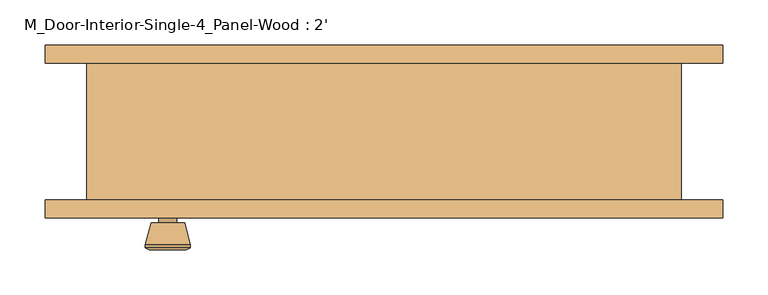
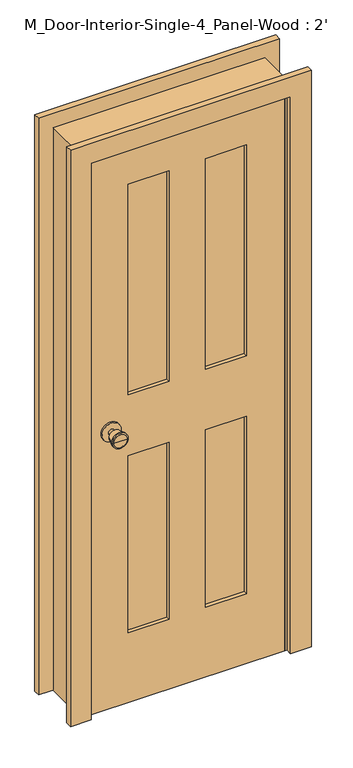
"""IFC4 building model written with IfcOpenShell, lengths in millimetres: door geometry, M_Door-Interior-Single-4_Panel-Wood : 2'."""

from ifc_helpers import new_model, si_unit, point, frame, frame_2d, origin, place, context, project, spatial, polyline, circle_curve, trimmed, segment, composite_curve, outline, extrude, faceted_brep, source, transform, mapped, element, save
from ifc_brep_helpers import plane_surface, cylinder_surface, revolved_surface, advanced_brep


def m_door_interior_single_4_panel_wood_2_b7882c25(model_context):
    return source(origin(), model_context, "Body", "SolidModel", [
        advanced_brep(
        [(-239.8, -32.025, 914.4), (-249.8, -32.025, 914.4), (-229.8, -32.025, 914.4), (-219.3241324, 16.975, 914.4), (-260.2758676, 16.975, 914.4), (-239.8, 16.975, 914.4), (-214.8, 15.1471319, 914.4), (-264.8, 15.1471319, 914.4), (-214.8, 11.6834537, 914.4), (-264.8, 11.6834537, 914.4), (-221.163764, -13.025, 914.4), (-258.436236, -13.025, 914.4), (-229.8, -13.025, 914.4), (-249.8, -13.025, 914.4)],
        [
            (0, 1),
            (1, 2, circle_curve(frame((-239.8, -32.025, 914.4), z_axis=(0.0, -1.0, 0.0), x_axis=(-1.0, 0.0, 0.0)), 10.0)),
            (2, 0),
            (2, 1, circle_curve(frame((-239.8, -32.025, 914.4), z_axis=(0.0, -1.0, 0.0), x_axis=(-1.0, 0.0, 0.0)), 10.0)),
            (3, 4, circle_curve(frame((-239.8, 16.975, 914.4), z_axis=(0.0, 1.0, 0.0), x_axis=(-1.0, 0.0, 0.0)), 20.4758676)),
            (4, 5),
            (5, 3),
            (4, 3, circle_curve(frame((-239.8, 16.975, 914.4), z_axis=(0.0, 1.0, 0.0), x_axis=(-1.0, 0.0, 0.0)), 20.4758676)),
            (6, 7, circle_curve(frame((-239.8, 15.1471319, 914.4), z_axis=(0.0, 1.0, 0.0), x_axis=(-1.0, 0.0, 0.0)), 25.0)),
            (7, 4),
            (3, 6),
            (7, 6, circle_curve(frame((-239.8, 15.1471319, 914.4), z_axis=(0.0, 1.0, 0.0), x_axis=(-1.0, 0.0, 0.0)), 25.0)),
            (8, 9, circle_curve(frame((-239.8, 11.6834537, 914.4), z_axis=(0.0, 1.0, 0.0), x_axis=(-1.0, 0.0, 0.0)), 25.0)),
            (9, 7),
            (6, 8),
            (9, 8, circle_curve(frame((-239.8, 11.6834537, 914.4), z_axis=(0.0, 1.0, 0.0), x_axis=(-1.0, 0.0, 0.0)), 25.0)),
            (10, 11, circle_curve(frame((-239.8, -13.025, 914.4), z_axis=(0.0, 1.0, 0.0), x_axis=(-1.0, 0.0, 0.0)), 18.636236)),
            (11, 9),
            (8, 10),
            (11, 10, circle_curve(frame((-239.8, -13.025, 914.4), z_axis=(0.0, 1.0, 0.0), x_axis=(-1.0, 0.0, 0.0)), 18.636236)),
            (12, 13, circle_curve(frame((-239.8, -13.025, 914.4), z_axis=(0.0, 1.0, 0.0), x_axis=(-1.0, 0.0, 0.0)), 10.0)),
            (13, 11),
            (10, 12),
            (13, 12, circle_curve(frame((-239.8, -13.025, 914.4), z_axis=(0.0, 1.0, 0.0), x_axis=(-1.0, 0.0, 0.0)), 10.0)),
            (1, 13),
            (12, 2),
        ],
        [
            plane_surface(frame((-239.8, -32.025, 914.4), z_axis=(0.0, -1.0, 0.0), x_axis=(-1.0, 0.0, 0.0))),
            plane_surface(frame((-239.8, 16.975, 914.4), z_axis=(0.0, 1.0, 0.0), x_axis=(-1.0, 0.0, 0.0))),
            revolved_surface(polyline([(-260.2758676, 16.975, 914.4), (-264.8, 15.1471319, 914.4)]), (-239.8, -32.025, 914.4), (0.0, -1.0, 0.0)),
            cylinder_surface(frame((-239.8, -32.025, 914.4), z_axis=(0.0, -1.0, 0.0), x_axis=(-1.0, 0.0, 0.0)), 25.0),
            revolved_surface(polyline([(-264.8, 11.6834537, 914.4), (-258.436236, -13.025, 914.4)]), (-239.8, -32.025, 914.4), (0.0, -1.0, 0.0)),
            plane_surface(frame((-239.8, -13.025, 914.4), z_axis=(0.0, -1.0, 0.0), x_axis=(-1.0, 0.0, 0.0))),
            cylinder_surface(frame((-239.8, -32.025, 914.4), z_axis=(0.0, -1.0, 0.0), x_axis=(-1.0, 0.0, 0.0)), 10.0),
        ],
        [
            (0, [[1, 2, 3]]),
            (0, [[-3, 4, -1]]),
            (1, [[5, 6, 7]]),
            (1, [[8, -7, -6]]),
            (2, [[9, 10, -5, 11]]),
            (2, [[12, -11, -8, -10]]),
            (3, [[13, 14, -9, 15]]),
            (3, [[16, -15, -12, -14]]),
            (4, [[17, 18, -13, 19]]),
            (4, [[20, -19, -16, -18]]),
            (5, [[21, 22, -17, 23]]),
            (5, [[24, -23, -20, -22]]),
            (6, [[-2, 25, -21, 26]]),
            (6, [[-4, -26, -24, -25]]),
        ],
    ),
        extrude(outline(composite_curve([segment(trimmed(circle_curve(frame_2d((914.4, -239.8)), 30.0), [point((914.4, -269.8))], [point((914.4, -209.8))], False, "CARTESIAN"), True, "CONTINUOUS"), segment(trimmed(circle_curve(frame_2d((914.4, -239.8)), 30.0), [point((914.4, -209.8))], [point((914.4, -269.8))], False, "CARTESIAN"), True, "CONTINUOUS")], self_intersect=False)), frame((0.0, -38.025, 0.0), z_axis=(0.0, 1.0, 0.0), x_axis=(0.0, 0.0, 1.0)), (0.0, 0.0, 1.0), 6.0),
        advanced_brep(
        [(-239.8, -79.025, 914.4), (-229.8, -79.025, 914.4), (-249.8, -79.025, 914.4), (-219.3241324, -128.025, 914.4), (-239.8, -128.025, 914.4), (-260.2758676, -128.025, 914.4), (-214.8, -126.1971319, 914.4), (-264.8, -126.1971319, 914.4), (-214.8, -122.7334537, 914.4), (-264.8, -122.7334537, 914.4), (-221.163764, -98.025, 914.4), (-258.436236, -98.025, 914.4), (-229.8, -98.025, 914.4), (-249.8, -98.025, 914.4)],
        [
            (0, 1),
            (1, 2, circle_curve(frame((-239.8, -79.025, 914.4), z_axis=(0.0, 1.0, 0.0), x_axis=(-1.0, 0.0, 0.0)), 10.0)),
            (2, 0),
            (2, 1, circle_curve(frame((-239.8, -79.025, 914.4), z_axis=(0.0, 1.0, 0.0), x_axis=(-1.0, 0.0, 0.0)), 10.0)),
            (3, 4),
            (4, 5),
            (5, 3, circle_curve(frame((-239.8, -128.025, 914.4), z_axis=(0.0, -1.0, 0.0), x_axis=(-1.0, 0.0, 0.0)), 20.4758676)),
            (3, 5, circle_curve(frame((-239.8, -128.025, 914.4), z_axis=(0.0, -1.0, 0.0), x_axis=(-1.0, 0.0, 0.0)), 20.4758676)),
            (6, 3),
            (5, 7),
            (7, 6, circle_curve(frame((-239.8, -126.1971319, 914.4), z_axis=(0.0, -1.0, 0.0), x_axis=(-1.0, 0.0, 0.0)), 25.0)),
            (6, 7, circle_curve(frame((-239.8, -126.1971319, 914.4), z_axis=(0.0, -1.0, 0.0), x_axis=(-1.0, 0.0, 0.0)), 25.0)),
            (8, 6),
            (7, 9),
            (9, 8, circle_curve(frame((-239.8, -122.7334537, 914.4), z_axis=(0.0, -1.0, 0.0), x_axis=(-1.0, 0.0, 0.0)), 25.0)),
            (8, 9, circle_curve(frame((-239.8, -122.7334537, 914.4), z_axis=(0.0, -1.0, 0.0), x_axis=(-1.0, 0.0, 0.0)), 25.0)),
            (10, 8),
            (9, 11),
            (11, 10, circle_curve(frame((-239.8, -98.025, 914.4), z_axis=(0.0, -1.0, 0.0), x_axis=(-1.0, 0.0, 0.0)), 18.636236)),
            (10, 11, circle_curve(frame((-239.8, -98.025, 914.4), z_axis=(0.0, -1.0, 0.0), x_axis=(-1.0, 0.0, 0.0)), 18.636236)),
            (12, 10),
            (11, 13),
            (13, 12, circle_curve(frame((-239.8, -98.025, 914.4), z_axis=(0.0, -1.0, 0.0), x_axis=(-1.0, 0.0, 0.0)), 10.0)),
            (12, 13, circle_curve(frame((-239.8, -98.025, 914.4), z_axis=(0.0, -1.0, 0.0), x_axis=(-1.0, 0.0, 0.0)), 10.0)),
            (1, 12),
            (13, 2),
        ],
        [
            plane_surface(frame((-239.8, -79.025, 914.4), z_axis=(0.0, 1.0, 0.0), x_axis=(-1.0, 0.0, 0.0))),
            plane_surface(frame((-239.8, -128.025, 914.4), z_axis=(0.0, -1.0, 0.0), x_axis=(-1.0, 0.0, 0.0))),
            revolved_surface(polyline([(-260.2758676, -128.025, 914.4), (-264.8, -126.1971319, 914.4)]), (-239.8, -79.025, 914.4), (0.0, 1.0, 0.0)),
            cylinder_surface(frame((-239.8, -79.025, 914.4), z_axis=(0.0, 1.0, 0.0), x_axis=(-1.0, 0.0, 0.0)), 25.0),
            revolved_surface(polyline([(-264.8, -122.7334537, 914.4), (-258.436236, -98.025, 914.4)]), (-239.8, -79.025, 914.4), (0.0, 1.0, 0.0)),
            plane_surface(frame((-239.8, -98.025, 914.4), z_axis=(0.0, 1.0, 0.0), x_axis=(-1.0, 0.0, 0.0))),
            cylinder_surface(frame((-239.8, -79.025, 914.4), z_axis=(0.0, 1.0, 0.0), x_axis=(-1.0, 0.0, 0.0)), 10.0),
        ],
        [
            (0, [[1, 2, 3]]),
            (0, [[-3, 4, -1]]),
            (1, [[5, 6, 7]]),
            (1, [[-6, -5, 8]]),
            (2, [[9, -7, 10, 11]]),
            (2, [[-10, -8, -9, 12]]),
            (3, [[13, -11, 14, 15]]),
            (3, [[-14, -12, -13, 16]]),
            (4, [[17, -15, 18, 19]]),
            (4, [[-18, -16, -17, 20]]),
            (5, [[21, -19, 22, 23]]),
            (5, [[-22, -20, -21, 24]]),
            (6, [[25, -23, 26, -2]]),
            (6, [[-26, -24, -25, -4]]),
        ],
    ),
        extrude(outline(composite_curve([segment(trimmed(circle_curve(frame_2d((914.4, -239.8)), 30.0), [point((914.4, -269.8))], [point((914.4, -209.8))], False, "CARTESIAN"), True, "CONTINUOUS"), segment(trimmed(circle_curve(frame_2d((914.4, -239.8)), 30.0), [point((914.4, -209.8))], [point((914.4, -269.8))], False, "CARTESIAN"), True, "CONTINUOUS")], self_intersect=False)), frame((0.0, -79.025, 0.0), z_axis=(0.0, 1.0, 0.0), x_axis=(0.0, 0.0, 1.0)), (0.0, 0.0, 1.0), 6.0),
        faceted_brep([(329.8, -73.025, 0.0), (304.8, -73.025, 0.0), (304.8, -38.025, 0.0), (292.1, -38.025, 0.0), (292.1, -3.1, 0.0), (304.8, -3.1, 0.0), (304.8, 79.375, 0.0), (329.8, 79.375, 0.0), (329.8, 79.375, 1853.8), (329.8, -73.025, 1853.8), (304.8, 79.375, 1828.8), (-304.8, 79.375, 1828.8), (-304.8, 79.375, 0.0), (-329.8, 79.375, 0.0), (-329.8, 79.375, 1853.8), (304.8, -3.1, 1828.8), (292.1, -3.1, 1816.1), (-292.1, -3.1, 1816.1), (-292.1, -3.1, 0.0), (-304.8, -3.1, 0.0), (-304.8, -3.1, 1828.8), (292.1, -38.025, 1816.1), (304.8, -38.025, 1828.8), (-304.8, -38.025, 1828.8), (-304.8, -38.025, 0.0), (-292.1, -38.025, 0.0), (-292.1, -38.025, 1816.1), (304.8, -73.025, 1828.8), (-329.8, -73.025, 1853.8), (-329.8, -73.025, 0.0), (-304.8, -73.025, 0.0), (-304.8, -73.025, 1828.8)], [[[0, 1, 2, 3, 4, 5, 6, 7]], [[7, 8, 9, 0]], [[6, 10, 11, 12, 13, 14, 8, 7]], [[5, 15, 10, 6]], [[4, 16, 17, 18, 19, 20, 15, 5]], [[3, 21, 16, 4]], [[2, 22, 23, 24, 25, 26, 21, 3]], [[1, 27, 22, 2]], [[0, 9, 28, 29, 30, 31, 27, 1]], [[8, 14, 28, 9]], [[15, 20, 11, 10]], [[21, 26, 17, 16]], [[27, 31, 23, 22]], [[29, 13, 12, 19, 18, 25, 24, 30]], [[14, 13, 29, 28]], [[20, 19, 12, 11]], [[26, 25, 18, 17]], [[31, 30, 24, 23]]]),
        extrude(outline(polyline([(1828.8, -304.8), (0.0, -304.8), (0.0, 304.8), (1828.8, 304.8), (1828.8, -304.8)]), holes=[polyline([(1708.8, 57.5), (1708.8, 184.8), (1014.4, 184.8), (1014.4, 57.5), (1708.8, 57.5)]), polyline([(1014.4, -57.5), (1014.4, -184.8), (1708.8, -184.8), (1708.8, -57.5), (1014.4, -57.5)]), polyline([(814.4, 57.5), (814.4, 184.8), (230.0, 184.8), (230.0, 57.5), (814.4, 57.5)]), polyline([(230.0, -57.5), (230.0, -184.8), (814.4, -184.8), (814.4, -57.5), (230.0, -57.5)])]), frame((0.0, -73.025, 0.0), z_axis=(0.0, 1.0, 0.0), x_axis=(0.0, 0.0, 1.0)), (0.0, 0.0, 1.0), 35.0),
        extrude(outline(polyline([(184.8, -49.6916667), (184.8, -61.3583333), (57.5, -61.3583333), (57.5, -49.6916667), (184.8, -49.6916667)])), frame((0.0, 0.0, 1014.4), z_axis=(0.0, 0.0, 1.0), x_axis=(1.0, 0.0, 0.0)), (0.0, 0.0, 1.0), 694.4),
        extrude(outline(polyline([(-57.5, -49.6916667), (-57.5, -61.3583333), (-184.8, -61.3583333), (-184.8, -49.6916667), (-57.5, -49.6916667)])), frame((0.0, 0.0, 1014.4), z_axis=(0.0, 0.0, 1.0), x_axis=(1.0, 0.0, 0.0)), (0.0, 0.0, 1.0), 694.4),
        extrude(outline(polyline([(184.8, -49.6916667), (184.8, -61.3583333), (57.5, -61.3583333), (57.5, -49.6916667), (184.8, -49.6916667)])), frame((0.0, 0.0, 230.0), z_axis=(0.0, 0.0, 1.0), x_axis=(1.0, 0.0, 0.0)), (0.0, 0.0, 1.0), 584.4),
        extrude(outline(polyline([(-57.5, -49.6916667), (-57.5, -61.3583333), (-184.8, -61.3583333), (-184.8, -49.6916667), (-57.5, -49.6916667)])), frame((0.0, 0.0, 230.0), z_axis=(0.0, 0.0, 1.0), x_axis=(1.0, 0.0, 0.0)), (0.0, 0.0, 1.0), 584.4),
        extrude(outline(polyline([(0.0, 376.15), (1900.15, 376.15), (1900.15, -376.15), (0.0, -376.15), (0.0, -311.15), (1835.15, -311.15), (1835.15, 311.15), (0.0, 311.15), (0.0, 376.15)])), frame((0.0, -93.025, 0.0), z_axis=(0.0, 1.0, 0.0), x_axis=(0.0, 0.0, 1.0)), (0.0, 0.0, 1.0), 20.0),
        extrude(outline(polyline([(0.0, 376.15), (1900.15, 376.15), (1900.15, -376.15), (0.0, -376.15), (0.0, -311.15), (1835.15, -311.15), (1835.15, 311.15), (0.0, 311.15), (0.0, 376.15)])), frame((0.0, 79.375, 0.0), z_axis=(0.0, 1.0, 0.0), x_axis=(0.0, 0.0, 1.0)), (0.0, 0.0, 1.0), 20.0),
    ])


if __name__ == "__main__":
    model = new_model("IFC4")
    model_context = context("Model", 3, world=origin())
    ifc_project = project(units=[si_unit("LENGTHUNIT", "METRE", prefix="MILLI")], contexts=[model_context])
    site = spatial("IfcSite", under=ifc_project)
    building = spatial("IfcBuilding", under=site)
    placement = place(None, origin())
    m_door_interior_single_4_panel_wood_2_shape = m_door_interior_single_4_panel_wood_2_b7882c25(model_context)
    element("IfcDoor", 1, ObjectType="M_Door-Interior-Single-4_Panel-Wood : 2'", at=placement, inside=building, context=model_context, shape_type="MappedRepresentation", body=[
        mapped(m_door_interior_single_4_panel_wood_2_shape, transform((0.0, 0.0, 0.0), x_axis=(1.0, 0.0, 0.0), y_axis=(0.0, 1.0, 0.0), z_axis=(0.0, 0.0, 1.0))),
    ])
    save(model, "model.ifc")

# Revit data of these elements
# Type "M_Door-Interior-Single-4_Panel-Wood : 2'"
#   Type Mark = "13"
#   Assembly Code = "C1020300"
#   Analytic Construction = "Wooden"
#   Top Rail = 0' - 4.72441"
#   Thickness = 0' - 1.37795"
#   Thermal Resistance (R) = 2.5876 (h·ft²·°F)/BTU
#   Swing Angle [instance default] = 90.00°
#   Stiles = 0' - 4.72441"
#   Rough Width = 2' - 1.9685"
#   Rough Height = 6' - 0.98425"
#   Mullion = 0' - 4.52756"
#   Lock Rail = 0' - 7.87402"
#   Height = 6' - 0"
#   Width = 2' - 0"
#   Heat Transfer Coefficient (U) = 0.3865 BTU/(h·ft²·°F)
#   Bottom Rail = 0' - 9.05512"
#   Trim Material = Cherry
#   Panel Material = Cherry
#   Frame Material = Cherry
#   Door Handle Material = Aluminum
#   Visual Light Transmittance = 0
#   Solar Heat Gain Coefficient = 0
#   Wall Closure = (empty or 0)
#   Function = (empty or 0)
# Element 1 (IfcDoor, "M_Door-Interior-Single-4_Panel-Wood : 2'")
#   Materials on its faces: "Cherry", "Aluminum"
# Materials
#   "Cherry": class "Wood", colour RGB 226 177 128, transparency 0, Description = "Prunus Serotina", Cost = 0
#   "Aluminum": class "Metal", colour RGB 247 247 247, transparency 0, Description = "Aluminum 6061", Cost = 0
